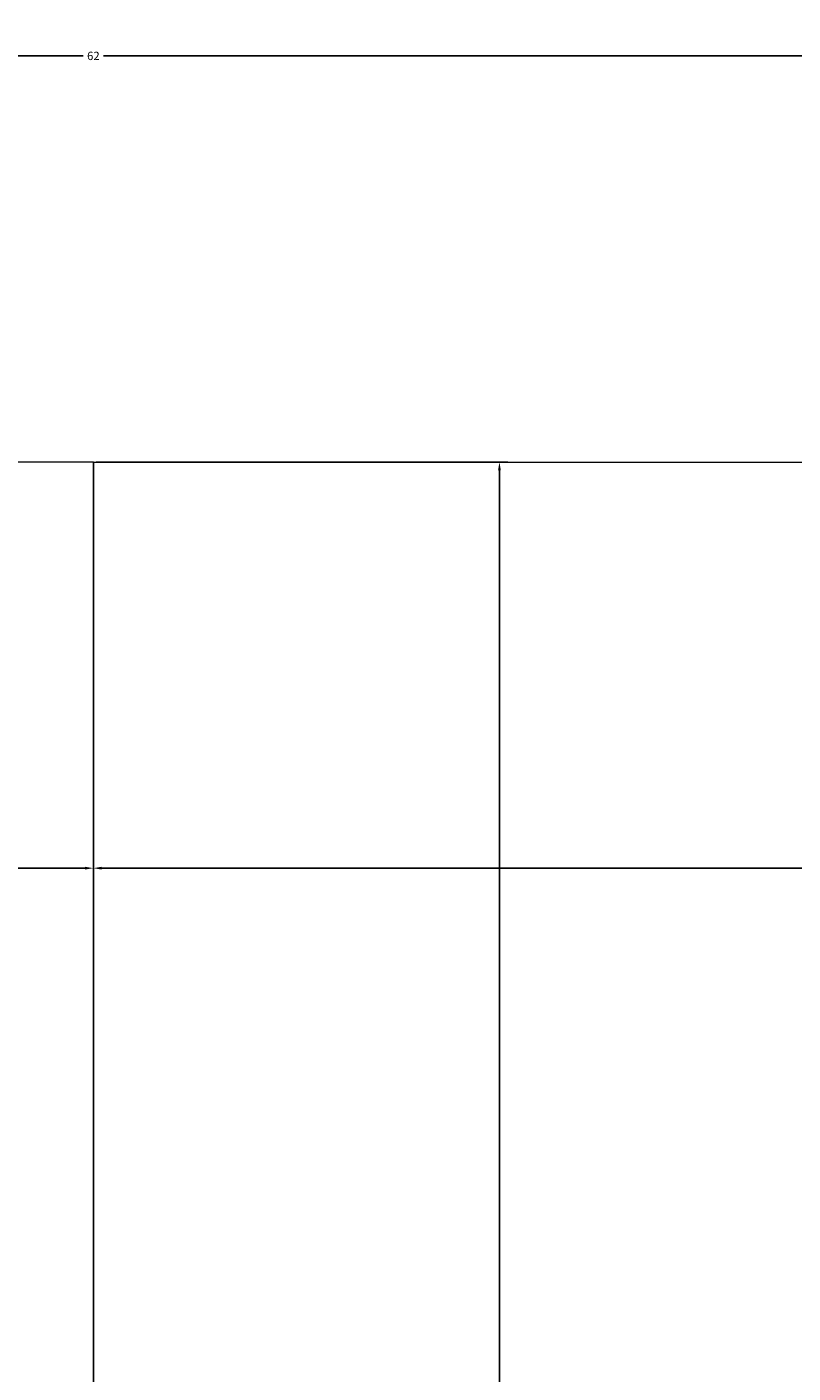
# Model space of a CAD drawing. Units: millimetres. Extents: x -9 to 135, y -119 to 27.
# Tile 7 of 12: x 62 to 78, y -18 to 11. Entities that reach past the tile are written whole.
import ezdxf

# ---------------------------------------------------------------- set-up
doc = ezdxf.new("R2010")
doc.units = ezdxf.units.MM
doc.layers.add('M-CONS', color=8, linetype='Continuous', lineweight=18)
doc.layers.add('M-DIMS', color=2, linetype='Continuous', lineweight=18)
doc.styles.get("Standard").update_dxf_attribs({"font": 'arial.ttf'})
doc.dimstyles.get("Standard").update_dxf_attribs({"dimtxt": 0.18, "dimasz": 0.18, "dimexe": 0.18, "dimexo": 0.0625, "dimgap": 0.09, "dimtad": 0, "dimtih": 1, "dimtoh": 1, "dimdec": 4, "dimzin": 0, "dimdsep": 46, "dimtxsty": 'Standard', "dimcen": 0.09, "dimadec": 0, "dimazin": 0, "dimtfac": 1, "dimtdec": 4, "dimtofl": 0, "dimtmove": 0, "dimatfit": 3, "dimfxl": 1, "dimtolj": 1, "dimtzin": 0, "dimarcsym": 0})

# ---------------------------------------------------------------- blocks, each defined once
blk = doc.blocks.new('*D2')
at = {"layer": 'Defpoints', "color": 0, "transparency": 16777216}
for p in [(126, 26.533), (0, 17.733), (126, 1.733)]:
    blk.add_point(p, dxfattribs=at)
at = {"layer": 'M-DIMS', "color": 0, "lineweight": -2, "transparency": 16777216}
for p, q in [((0, 17.796), (0, 26.713)), ((126, 1.796), (126, 26.713)), ((0.18, 26.533), (62.72, 26.533)), ((125.82, 26.533), (63.28, 26.533))]:
    blk.add_line(p, q, dxfattribs=at)
at = {"layer": 'M-DIMS', "color": 0, "transparency": 16777216}
for points in [[(0.18, 26.563), (0.18, 26.503), (0, 26.533)], [(125.82, 26.563), (125.82, 26.503), (126, 26.533)]]:
    blk.add_solid(points, dxfattribs=at)
at = {"layer": 'M-DIMS', "color": 0, "transparency": 16777216, "insert": (63, 26.533), "char_height": 0.18, "attachment_point": 5}
blk.add_mtext('\\A1;126', dxfattribs=at)
blk = doc.blocks.new('*D3')
at = {"layer": 'Defpoints', "color": 0, "transparency": 16777216}
for p in [(0, 17.733), (-8.8, -110.267), (63, -110.267)]:
    blk.add_point(p, dxfattribs=at)
at = {"layer": 'M-DIMS', "color": 0, "lineweight": -2, "transparency": 16777216}
for p, q in [((-0.062, 17.733), (-8.98, 17.733)), ((-8.8, 17.553), (-8.8, -46.085)), ((-8.8, -110.087), (-8.8, -46.449)), ((62.938, -110.267), (-8.98, -110.267))]:
    blk.add_line(p, q, dxfattribs=at)
at = {"layer": 'M-DIMS', "color": 0, "transparency": 16777216}
for points in [[(-8.83, 17.553), (-8.77, 17.553), (-8.8, 17.733)], [(-8.83, -110.087), (-8.77, -110.087), (-8.8, -110.267)]]:
    blk.add_solid(points, dxfattribs=at)
at = {"layer": 'M-DIMS', "color": 0, "transparency": 16777216, "insert": (-8.8, -46.267), "char_height": 0.18, "attachment_point": 5}
blk.add_mtext('\\A1;128', dxfattribs=at)
blk = doc.blocks.new('*D6')
at = {"layer": 'Defpoints', "color": 0, "transparency": 16777216}
for p in [(94, 10.533), (32, 1.733), (94, 1.733)]:
    blk.add_point(p, dxfattribs=at)
at = {"layer": 'M-DIMS', "color": 0, "lineweight": -2, "transparency": 16777216}
for p, q in [((32, 1.796), (32, 10.713)), ((32.18, 10.533), (62.782, 10.533)), ((93.82, 10.533), (63.218, 10.533)), ((94, 1.796), (94, 10.713))]:
    blk.add_line(p, q, dxfattribs=at)
at = {"layer": 'M-DIMS', "color": 0, "transparency": 16777216}
for points in [[(32.18, 10.563), (32.18, 10.503), (32, 10.533)], [(93.82, 10.563), (93.82, 10.503), (94, 10.533)]]:
    blk.add_solid(points, dxfattribs=at)
at = {"layer": 'M-DIMS', "color": 0, "transparency": 16777216, "insert": (63, 10.533), "char_height": 0.18, "attachment_point": 5}
blk.add_mtext('\\A1;62', dxfattribs=at)
blk = doc.blocks.new('*D9')
at = {"layer": 'Defpoints', "color": 0, "transparency": 16777216}
for p in [(32, 1.733), (63, 1.733), (32, -7.067)]:
    blk.add_point(p, dxfattribs=at)
at = {"layer": 'M-DIMS', "color": 0, "lineweight": -2, "transparency": 16777216}
for p, q in [((32, 1.671), (32, -7.247)), ((63, 1.671), (63, -7.247)), ((32.18, -7.067), (47.299, -7.067)), ((62.82, -7.067), (47.701, -7.067))]:
    blk.add_line(p, q, dxfattribs=at)
at = {"layer": 'M-DIMS', "color": 0, "transparency": 16777216}
for points in [[(32.18, -7.037), (32.18, -7.097), (32, -7.067)], [(62.82, -7.037), (62.82, -7.097), (63, -7.067)]]:
    blk.add_solid(points, dxfattribs=at)
at = {"layer": 'M-DIMS', "color": 0, "transparency": 16777216, "insert": (47.5, -7.067), "char_height": 0.18, "attachment_point": 5}
blk.add_mtext('\\A1;31', dxfattribs=at)
blk = doc.blocks.new('*D10')
at = {"layer": 'Defpoints', "color": 0, "transparency": 16777216}
for p in [(63, 1.733), (108, 1.733), (63, -7.067)]:
    blk.add_point(p, dxfattribs=at)
at = {"layer": 'M-DIMS', "color": 0, "lineweight": -2, "transparency": 16777216}
for p, q in [((63, 1.671), (63, -7.247)), ((108, 1.671), (108, -7.247)), ((63.18, -7.067), (85.277, -7.067)), ((107.82, -7.067), (85.723, -7.067))]:
    blk.add_line(p, q, dxfattribs=at)
at = {"layer": 'M-DIMS', "color": 0, "transparency": 16777216}
for points in [[(63.18, -7.037), (63.18, -7.097), (63, -7.067)], [(107.82, -7.037), (107.82, -7.097), (108, -7.067)]]:
    blk.add_solid(points, dxfattribs=at)
at = {"layer": 'M-DIMS', "color": 0, "transparency": 16777216, "insert": (85.5, -7.067), "char_height": 0.18, "attachment_point": 5}
blk.add_mtext('\\A1;45', dxfattribs=at)
blk = doc.blocks.new('*D12')
at = {"layer": 'Defpoints', "color": 0, "transparency": 16777216}
for p in [(63, 1.733), (63, -61.267), (71.8, -61.267)]:
    blk.add_point(p, dxfattribs=at)
at = {"layer": 'M-DIMS', "color": 0, "lineweight": -2, "transparency": 16777216}
for p, q in [((63.063, 1.733), (71.98, 1.733)), ((71.8, 1.553), (71.8, -29.585)), ((71.8, -61.087), (71.8, -29.949)), ((63.063, -61.267), (71.98, -61.267))]:
    blk.add_line(p, q, dxfattribs=at)
at = {"layer": 'M-DIMS', "color": 0, "transparency": 16777216}
for points in [[(71.77, 1.553), (71.83, 1.553), (71.8, 1.733)], [(71.77, -61.087), (71.83, -61.087), (71.8, -61.267)]]:
    blk.add_solid(points, dxfattribs=at)
at = {"layer": 'M-DIMS', "color": 0, "transparency": 16777216, "insert": (71.8, -29.767), "char_height": 0.18, "attachment_point": 5}
blk.add_mtext('\\A1;63', dxfattribs=at)
blk = doc.blocks.new('*D13')
at = {"layer": 'Defpoints', "color": 0, "transparency": 16777216}
for p in [(126, 1.733), (63, -92.267), (134.8, -92.267)]:
    blk.add_point(p, dxfattribs=at)
at = {"layer": 'M-DIMS', "color": 0, "lineweight": -2, "transparency": 16777216}
for p, q in [((126.062, 1.733), (134.98, 1.733)), ((134.8, 1.553), (134.8, -45.085)), ((134.8, -92.087), (134.8, -45.449)), ((63.063, -92.267), (134.98, -92.267))]:
    blk.add_line(p, q, dxfattribs=at)
at = {"layer": 'M-DIMS', "color": 0, "transparency": 16777216}
for points in [[(134.77, 1.553), (134.83, 1.553), (134.8, 1.733)], [(134.77, -92.087), (134.83, -92.087), (134.8, -92.267)]]:
    blk.add_solid(points, dxfattribs=at)
at = {"layer": 'M-DIMS', "color": 0, "transparency": 16777216, "insert": (134.8, -45.267), "char_height": 0.18, "attachment_point": 5}
blk.add_mtext('\\A1;94', dxfattribs=at)
blk = doc.blocks.new('*D16')
at = {"layer": 'Defpoints', "color": 0, "transparency": 16777216}
for p in [(126, 1.733), (63, -92.267), (126, -119.067)]:
    blk.add_point(p, dxfattribs=at)
at = {"layer": 'M-DIMS', "color": 0, "lineweight": -2, "transparency": 16777216}
for p, q in [((126, 1.671), (126, -119.247)), ((63, -92.329), (63, -119.247)), ((63.18, -119.067), (94.281, -119.067)), ((125.82, -119.067), (94.719, -119.067))]:
    blk.add_line(p, q, dxfattribs=at)
at = {"layer": 'M-DIMS', "color": 0, "transparency": 16777216}
for points in [[(63.18, -119.037), (63.18, -119.097), (63, -119.067)], [(125.82, -119.037), (125.82, -119.097), (126, -119.067)]]:
    blk.add_solid(points, dxfattribs=at)
at = {"layer": 'M-DIMS', "color": 0, "transparency": 16777216, "insert": (94.5, -119.067), "char_height": 0.18, "attachment_point": 5}
blk.add_mtext('\\A1;63', dxfattribs=at)

msp = doc.modelspace()

# ---------------------------------------------------------------- linework, layer by layer
at = {"layer": 'M-CONS'}
for q in [(32, 1.733, 115.129), (94, 1.733, 115.129)]:
    msp.add_line((63, 1.733, 115.129), q, dxfattribs=at)
msp.add_polyline3d([(63, 1.733, 115.129), (63, -61.267, 115.129), (63, 1.733, 71.129)], close=True, dxfattribs=at)

# ---------------------------------------------------------------- dimensions: what is measured, and where the dimension line sits
at = {"layer": 'M-DIMS'}
for base, p1, p2, picture, middle in [((126, 26.533), (0, 17.733), (126, 1.733), '*D2', (63, 26.533)), ((94, 10.533), (32, 1.733), (94, 1.733), '*D6', (63, 10.533)), ((126, -119.067), (63, -92.267), (126, 1.733), '*D16', (94.5, -119.067))]:
    dim = msp.add_linear_dim(base=base, p1=p1, p2=p2, dimstyle='Standard', override={"dimdec": 0, "dimlfac": 1, "dimrnd": 0, "dimzin": 0, "dimdsep": 46, "dimlunit": 2}, dxfattribs=at)
    dim.commit()
    dim.dimension.update_dxf_attribs({"geometry": picture, "text_midpoint": middle})
for base, p1, p2, angle, picture, middle in [((-8.8, -110.267), (0, 17.733), (63, -110.267), 90, '*D3', (-8.8, -46.267)), ((32, -7.067), (63, 1.733), (32, 1.733), 180, '*D9', (47.5, -7.067)), ((63, -7.067), (108, 1.733), (63, 1.733), 180, '*D10', (85.5, -7.067)), ((71.8, -61.267), (63, 1.733), (63, -61.267), 270, '*D12', (71.8, -29.767)), ((134.8, -92.267), (126, 1.733), (63, -92.267), 90, '*D13', (134.8, -45.267))]:
    dim = msp.add_linear_dim(base=base, p1=p1, p2=p2, angle=angle, dimstyle='Standard', override={"dimdec": 0, "dimlfac": 1, "dimrnd": 0, "dimzin": 0, "dimdsep": 46, "dimlunit": 2}, dxfattribs=at)
    dim.commit()
    dim.dimension.update_dxf_attribs({"geometry": picture, "text_midpoint": middle})

doc.saveas('drawing.dxf')
